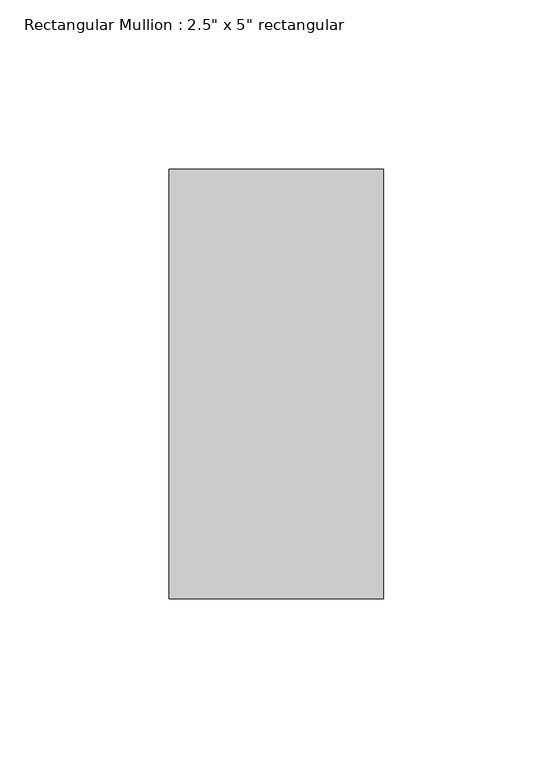
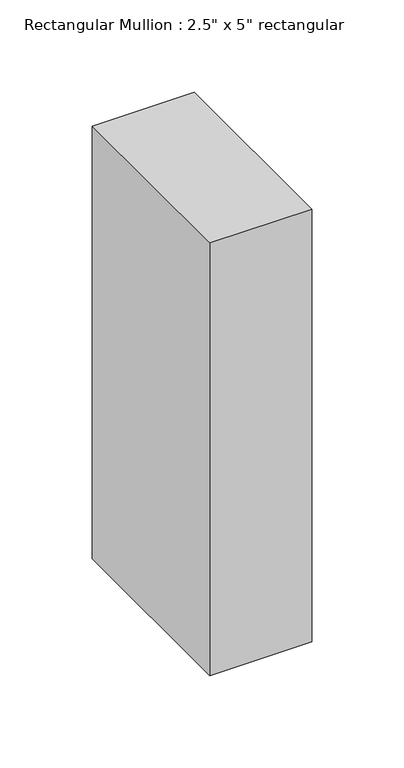
"""IFC4 building model written with IfcOpenShell, lengths in millimetres: member geometry."""

from ifc_helpers import new_model, si_unit, frame, origin, place, context, project, spatial, polyline, outline, extrude, source, transform, mapped, element, save


def member_6c34f49c(model_context):
    return source(origin(), model_context, "Body", "SweptSolid", [
        extrude(outline(polyline([(0.0, 63.5), (0.0, -63.5), (-63.5, -63.5), (-63.5, 63.5), (0.0, 63.5)])), frame((0.0, 0.0, -285.75), z_axis=(0.0, 0.0, 1.0), x_axis=(1.0, 0.0, 0.0)), (0.0, 0.0, 1.0), 285.75),
    ])


if __name__ == "__main__":
    model = new_model("IFC4")
    model_context = context("Model", 3, world=origin())
    ifc_project = project(units=[si_unit("LENGTHUNIT", "METRE", prefix="MILLI")], contexts=[model_context])
    site = spatial("IfcSite", under=ifc_project)
    building = spatial("IfcBuilding", under=site)
    placement = place(None, origin())
    member_shape = member_6c34f49c(model_context)
    element("IfcMember", 1, ObjectType="Rectangular Mullion : 2.5\" x 5\" rectangular", at=placement, inside=building, context=model_context, shape_type="MappedRepresentation", body=[
        mapped(member_shape, transform((0.0, 0.0, 0.0), x_axis=(1.0, 0.0, 0.0), y_axis=(0.0, 1.0, 0.0), z_axis=(0.0, 0.0, 1.0))),
    ])
    save(model, "model.ifc")

# Revit data of these elements
# Type "Rectangular Mullion : 2.5\" x 5\" rectangular"
#   built-in parameter 1007304 = 0.416667 (stored number, unit not read)
#   built-in parameter 1007301 = 0.104167 (stored number, unit not read)
#   built-in parameter 1007300 = 0.104167 (stored number, unit not read)
